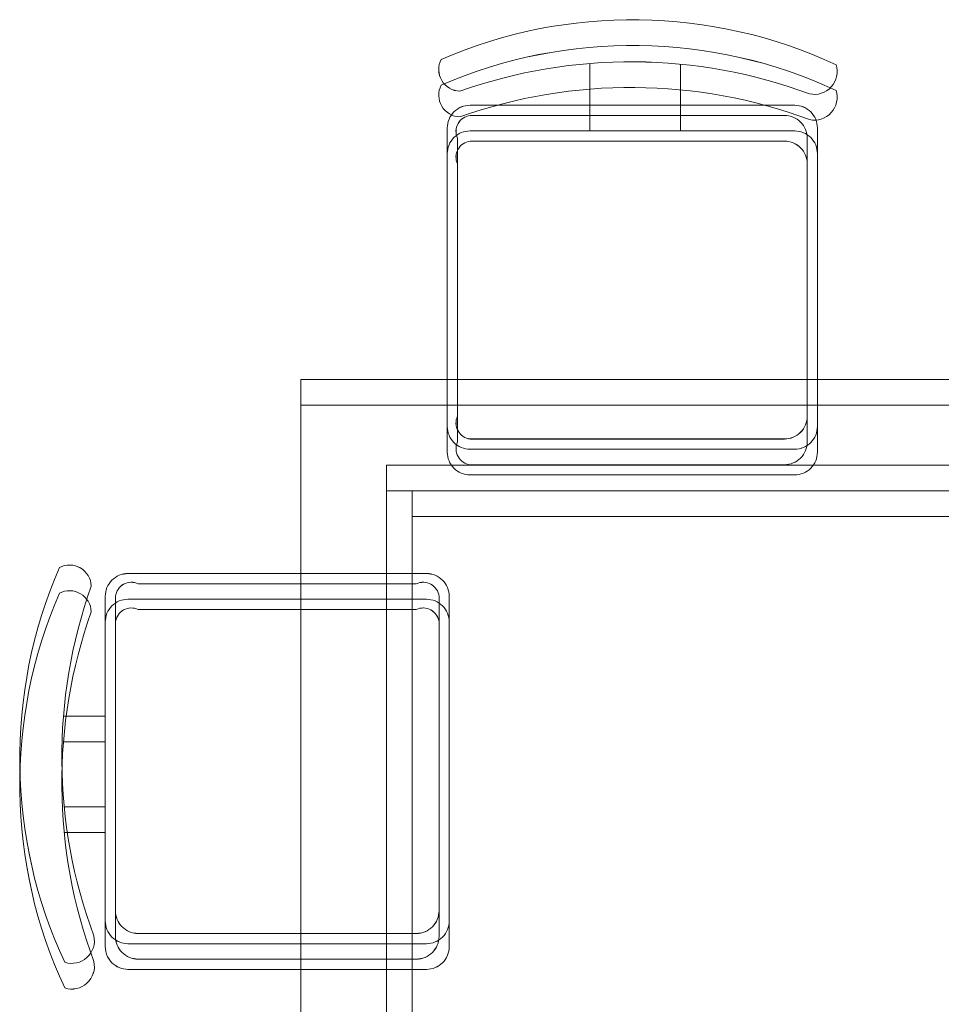
# Model space of a CAD drawing. Units: inches. Extents: x 1885 to 2748, y 783 to 2421.
# Tile 24 of 117: x 2340 to 2367, y 1261 to 1290. Entities that reach past the tile are written whole.
import ezdxf

# ---------------------------------------------------------------- set-up
doc = ezdxf.new("R2010")
doc.units = ezdxf.units.IN
doc.layers.add('A-FURN', color=8, linetype='Continuous', lineweight=13)

# ---------------------------------------------------------------- blocks, each defined once
blk = doc.blocks.new('TABLE-DINING-RECT')
for points in [[(-0.004, 23.421), (37.776, 23.421), (37.776, 0.754), (-0.004, 0.754)], [(-0.004, 23.421), (37.776, 23.421), (37.776, 0.753), (-0.004, 0.753)], [(-0.004, 22.666), (37.776, 22.666), (37.776, -0.002), (-0.004, -0.002)], [(-0.004, 22.665), (37.776, 22.665), (37.776, -0.002), (-0.004, -0.002)], [(2.515, 20.903), (35.257, 20.903), (35.257, 3.272), (2.515, 3.272)], [(2.515, 20.902), (35.257, 20.902), (35.257, 3.272), (2.515, 3.272)], [(2.515, 20.147), (35.257, 20.147), (35.257, 2.517), (2.515, 2.517)], [(2.515, 20.147), (35.257, 20.147), (35.257, 2.516), (2.515, 2.516)], [(3.27, 20.147), (34.501, 20.147), (34.501, 4.028), (3.27, 4.028)], [(3.27, 20.147), (34.501, 20.147), (34.501, 4.027), (3.27, 4.027)], [(3.27, 19.391), (34.501, 19.391), (34.501, 3.272), (3.27, 3.272)], [(3.27, 19.391), (34.501, 19.391), (34.501, 3.272), (3.27, 3.272)]]:
    blk.add_lwpolyline(points, close=True)

msp = doc.modelspace()

# ---------------------------------------------------------------- linework, layer by layer
at = {"layer": 'A-FURN'}
for points in [[(2353.309, 1288.172, -0.175809), (2363.599, 1288.094, 0.578392), (2364.379, 1288.951, 0.214524), (2352.763, 1289.107, 0.552014), (2353.309, 1288.172, -0.065079)], [(2353.309, 1288.171, -0.175809), (2363.599, 1288.094, 0.578392), (2364.379, 1288.951, 0.214524), (2352.763, 1289.107, 0.552014), (2353.309, 1288.171, -0.065079)], [(2353.309, 1287.416, -0.175809), (2363.599, 1287.338, 0.578392), (2364.379, 1288.196, 0.214524), (2352.763, 1288.351, 0.552014), (2353.309, 1287.416, -0.065079)], [(2353.309, 1287.416, -0.175809), (2363.599, 1287.338, 0.578392), (2364.379, 1288.195, 0.214524), (2352.763, 1288.351, 0.552014), (2353.309, 1287.416, -0.065079)], [(2359.807, 1287.759), (2359.807, 1288.967, -0.064759)], [(2359.807, 1287.758), (2359.807, 1288.967, -0.064759)], [(2359.807, 1287.003), (2359.807, 1288.211, -0.064759)], [(2359.807, 1287.003), (2359.807, 1288.211, -0.064759)], [(2363.163, 1287.759), (2353.61, 1287.759, 0.414214), (2352.941, 1287.091), (2352.941, 1278.307, 0.414214), (2353.61, 1277.638), (2363.163, 1277.638, 0.414214), (2363.831, 1278.307), (2363.831, 1287.091, 0.414214), (2363.163, 1287.759)], [(2363.163, 1287.758), (2353.61, 1287.758, 0.414214), (2352.941, 1287.09), (2352.941, 1278.306, 0.414214), (2353.61, 1277.638), (2363.163, 1277.638, 0.414214), (2363.831, 1278.306), (2363.831, 1287.09, 0.414214), (2363.163, 1287.758)], [(2363.163, 1287.003), (2353.61, 1287.003, 0.414214), (2352.941, 1286.335), (2352.941, 1277.551, 0.414214), (2353.61, 1276.883), (2363.163, 1276.883, 0.414214), (2363.831, 1277.551), (2363.831, 1286.335, 0.414214), (2363.163, 1287.003)], [(2363.163, 1287.003), (2353.61, 1287.003, 0.414214), (2352.941, 1286.335), (2352.941, 1277.551, 0.414214), (2353.61, 1276.883), (2363.163, 1276.883, 0.414214), (2363.831, 1277.551), (2363.831, 1286.335, 0.414214), (2363.163, 1287.003)], [(2342.544, 1263.323, -0.578392), (2341.687, 1262.543, -0.214524), (2341.531, 1274.159, -0.552014), (2342.466, 1273.613, 0.175809), (2342.544, 1263.323)], [(2342.544, 1263.323, -0.578392), (2341.687, 1262.543, -0.214524), (2341.531, 1274.158, -0.552014), (2342.466, 1273.613, 0.175809), (2342.544, 1263.323)], [(2342.879, 1273.312, -0.414214), (2343.547, 1273.981), (2352.331, 1273.981, -0.414214), (2352.999, 1273.312), (2352.999, 1263.76, -0.414214), (2352.331, 1263.091), (2343.547, 1263.091, -0.414214), (2342.879, 1263.76), (2342.879, 1273.312)], [(2342.879, 1273.312, -0.414214), (2343.547, 1273.98), (2352.331, 1273.98, -0.414214), (2352.999, 1273.312), (2352.999, 1263.759, -0.414214), (2352.331, 1263.091), (2343.547, 1263.091, -0.414214), (2342.879, 1263.759), (2342.879, 1273.312)], [(2342.544, 1262.567, -0.578392), (2341.687, 1261.788, -0.214524), (2341.531, 1273.403, -0.552014), (2342.466, 1272.857, 0.175809), (2342.544, 1262.567)], [(2342.544, 1262.567, -0.578392), (2341.687, 1261.787, -0.214524), (2341.531, 1273.403, -0.552014), (2342.466, 1272.857, 0.175809), (2342.544, 1262.567)], [(2342.879, 1272.557, -0.414214), (2343.547, 1273.225), (2352.331, 1273.225, -0.414214), (2352.999, 1272.557), (2352.999, 1263.004, -0.414214), (2352.331, 1262.336), (2343.547, 1262.336, -0.414214), (2342.879, 1263.004), (2342.879, 1272.557)], [(2342.879, 1272.557, -0.414214), (2343.547, 1273.225), (2352.331, 1273.225, -0.414214), (2352.999, 1272.557), (2352.999, 1263.004, -0.414214), (2352.331, 1262.335), (2343.547, 1262.335, -0.414214), (2342.879, 1263.004), (2342.879, 1272.557)], [(2342.879, 1267.115), (2341.671, 1267.115, 0.064759)], [(2342.879, 1267.115), (2341.671, 1267.115, 0.064759)], [(2342.879, 1266.359), (2341.671, 1266.359, 0.064759)], [(2342.879, 1266.359), (2341.671, 1266.359, 0.064759)]]:
    msp.add_lwpolyline(points, format="xyb", dxfattribs=at)
for points in [[(2357.133, 1288.989), (2357.133, 1287.759)], [(2357.133, 1288.989), (2357.133, 1287.758)], [(2357.133, 1288.233), (2357.133, 1287.003)], [(2357.133, 1288.233), (2357.133, 1287.003)], [(2341.649, 1269.789), (2342.879, 1269.789)], [(2341.649, 1269.789), (2342.879, 1269.789)], [(2341.649, 1269.033), (2342.879, 1269.033)], [(2341.649, 1269.033), (2342.879, 1269.033)]]:
    msp.add_lwpolyline(points, dxfattribs=at)
for points in [[(2353.614, 1287.458), (2362.862, 1287.458, -0.414214), (2363.53, 1286.789), (2363.53, 1278.608, -0.414214), (2362.862, 1277.94), (2353.614, 1277.94, -0.512069), (2353.242, 1278.608), (2353.242, 1286.789, -0.512069)], [(2353.614, 1287.457), (2362.862, 1287.457, -0.414214), (2363.53, 1286.789), (2363.53, 1278.608, -0.414214), (2362.862, 1277.939), (2353.614, 1277.939, -0.512069), (2353.242, 1278.608), (2353.242, 1286.789, -0.512069)], [(2353.614, 1286.702), (2362.862, 1286.702, -0.414214), (2363.53, 1286.034), (2363.53, 1277.852, -0.414214), (2362.862, 1277.184), (2353.614, 1277.184, -0.512069), (2353.242, 1277.852), (2353.242, 1286.034, -0.512069)], [(2353.614, 1286.702), (2362.862, 1286.702, -0.414214), (2363.53, 1286.033), (2363.53, 1277.852, -0.414214), (2362.862, 1277.184), (2353.614, 1277.184, -0.512069), (2353.242, 1277.852), (2353.242, 1286.033, -0.512069)], [(2343.18, 1273.308), (2343.18, 1264.061, 0.414214), (2343.848, 1263.392), (2352.03, 1263.392, 0.414214), (2352.698, 1264.061), (2352.698, 1273.308, 0.512069), (2352.03, 1273.68), (2343.848, 1273.68, 0.512069)], [(2343.18, 1273.308), (2343.18, 1264.06, 0.414214), (2343.848, 1263.392), (2352.03, 1263.392, 0.414214), (2352.698, 1264.06), (2352.698, 1273.308, 0.512069), (2352.03, 1273.679), (2343.848, 1273.679, 0.512069)], [(2343.18, 1272.553), (2343.18, 1263.305, 0.414214), (2343.848, 1262.637), (2352.03, 1262.637, 0.414214), (2352.698, 1263.305), (2352.698, 1272.553, 0.512069), (2352.03, 1272.924), (2343.848, 1272.924, 0.512069)], [(2343.18, 1272.552), (2343.18, 1263.305, 0.414214), (2343.848, 1262.636), (2352.03, 1262.636, 0.414214), (2352.698, 1263.305), (2352.698, 1272.552, 0.512069), (2352.03, 1272.924), (2343.848, 1272.924, 0.512069)]]:
    msp.add_lwpolyline(points, format="xyb", close=True, dxfattribs=at)

# ---------------------------------------------------------------- block references
msp.add_blockref('TABLE-DINING-RECT', (2348.64, 1256.27), dxfattribs=at)

doc.saveas('drawing.dxf')
